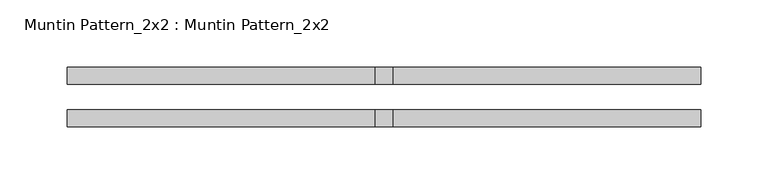
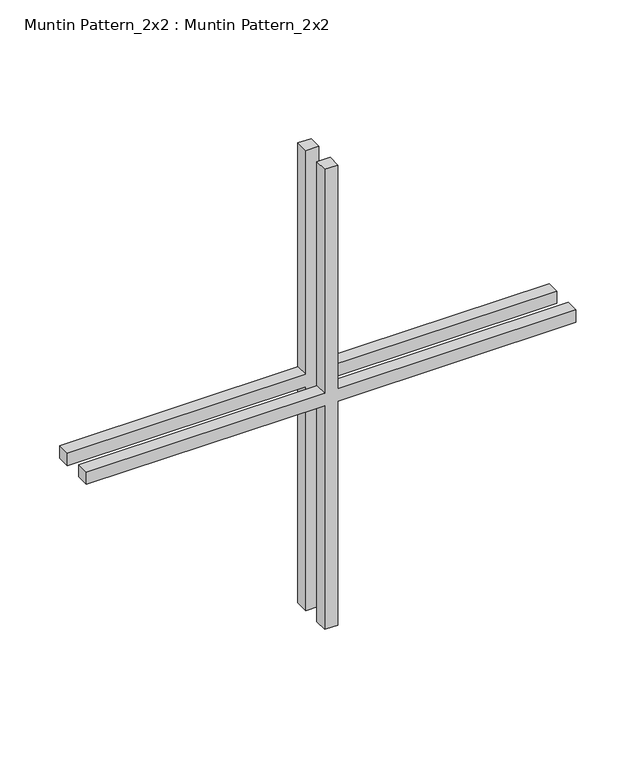
"""IFC4 building model written with IfcOpenShell, lengths in millimetres: proxy geometry, Muntin Pattern_2x2 : Muntin Pattern_2x2."""

from ifc_helpers import new_model, si_unit, frame, origin, place, context, project, spatial, polyline, outline, extrude, source, transform, mapped, element, save


def muntin_pattern_2x2_muntin_pattern_2x2_d662aa9d(model_context):
    return source(origin(), model_context, "Body", "SweptSolid", [
        extrude(outline(polyline([(241.3, -6.35), (241.3, -236.5375), (228.6, -236.5375), (228.6, -6.35), (0.0, -6.35), (0.0, 6.35), (228.6, 6.35), (228.6, 236.5375), (241.3, 236.5375), (241.3, 6.35), (469.9, 6.35), (469.9, -6.35), (241.3, -6.35)])), frame((0.0, -22.225, 0.0), z_axis=(0.0, 1.0, 0.0), x_axis=(0.0, 0.0, 1.0)), (0.0, 0.0, 1.0), 12.7),
        extrude(outline(polyline([(241.3, -6.35), (241.3, -236.5375), (228.6, -236.5375), (228.6, -6.35), (0.0, -6.35), (0.0, 6.35), (228.6, 6.35), (228.6, 236.5375), (241.3, 236.5375), (241.3, 6.35), (469.9, 6.35), (469.9, -6.35), (241.3, -6.35)])), frame((0.0, 9.525, 0.0), z_axis=(0.0, 1.0, 0.0), x_axis=(0.0, 0.0, 1.0)), (0.0, 0.0, 1.0), 12.7),
    ])


if __name__ == "__main__":
    model = new_model("IFC4")
    model_context = context("Model", 3, world=origin())
    ifc_project = project(units=[si_unit("LENGTHUNIT", "METRE", prefix="MILLI")], contexts=[model_context])
    site = spatial("IfcSite", under=ifc_project)
    building = spatial("IfcBuilding", under=site)
    placement = place(None, origin())
    muntin_pattern_2x2_muntin_pattern_2x2_shape = muntin_pattern_2x2_muntin_pattern_2x2_d662aa9d(model_context)
    element("IfcBuildingElementProxy", 1, Name="Muntin Pattern_2x2 : Muntin Pattern_2x2", ObjectType="Muntin Pattern_2x2 : Muntin Pattern_2x2", at=placement, inside=building, context=model_context, shape_type="MappedRepresentation", body=[
        mapped(muntin_pattern_2x2_muntin_pattern_2x2_shape, transform((0.0, 0.0, 0.0), x_axis=(1.0, 0.0, 0.0), y_axis=(0.0, 1.0, 0.0), z_axis=(0.0, 0.0, 1.0))),
    ])
    save(model, "model.ifc")

# Revit data of these elements
# Type "Muntin Pattern_2x2 : Muntin Pattern_2x2"
#   Width [instance default] = 4' - 0"
#   Thickness = 0' - 0 1/2"
#   Height [instance default] = 4' - 0"
#   Distance = 0' - 0 3/4"
#   Interior Material [instance default] = none
#   Exterior Material [instance default] = none
#   Default Elevation = 0
# Element 1 (IfcBuildingElementProxy, "Muntin Pattern_2x2 : Muntin Pattern_2x2")
#   Width = 1' - 6 5/8"
#   Height = 1' - 6 1/2"
#   Interior Material = Wood - Stained
#   Exterior Material = Clad - White
#   Materials on its faces: "Clad - White", "Wood - Stained"
# Materials
#   "Clad - White": class "Wood", colour RGB 242 242 238, transparency 0, Cost = 0
#   "Wood - Stained": class "Wood", colour RGB 224 178 126, transparency 0, Cost = 0
